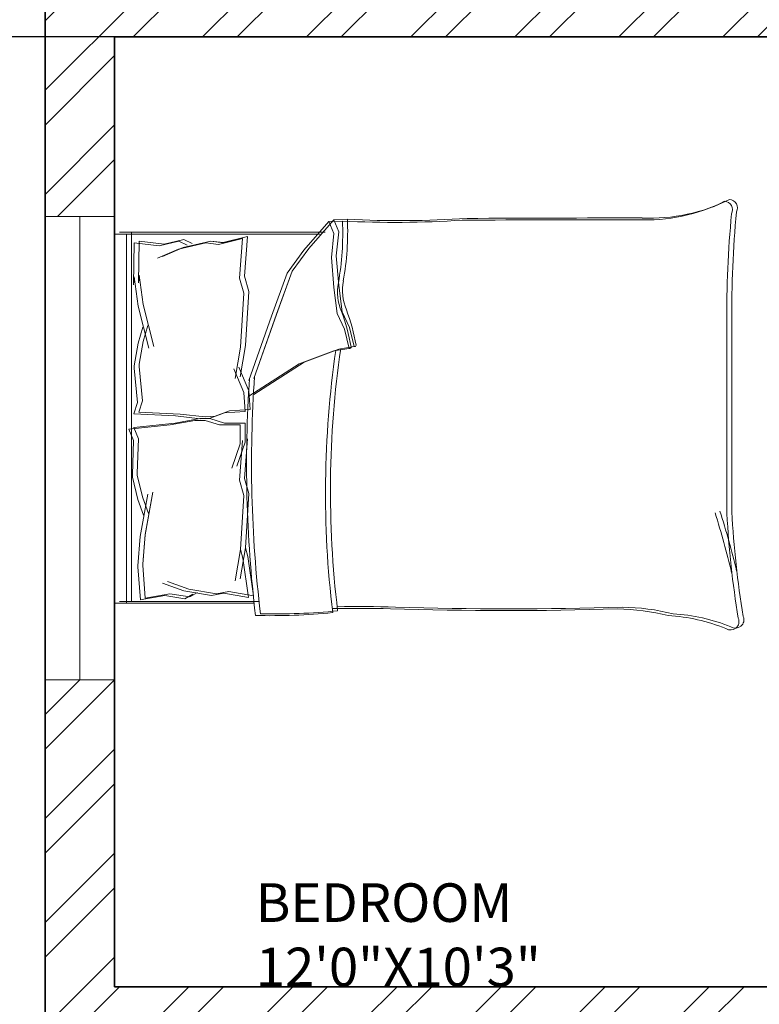
# Model space of a CAD drawing. Units: inches. Extents: x 2120 to 4013, y 1390 to 3019.
# Tile 5 of 59: x 2259 to 2355, y 1740 to 1868. Entities that reach past the tile are written whole.
import ezdxf

# ---------------------------------------------------------------- set-up
doc = ezdxf.new("R2010")
doc.units = ezdxf.units.IN
for name, color, linetype, lineweight in [('A-ANNO-DIMS', 2, 'Continuous', 18), ('A-AREA-IDEN', 7, 'Continuous', 18), ('A-FURN', 8, 'Continuous', 13), ('A-GLAZ', 4, 'Continuous', 18), ('A-WALL', 7, 'Continuous', 35), ('A-WALL-PATT', 252, 'Continuous', 13)]:
    doc.layers.add(name, color=color, linetype=linetype, lineweight=lineweight)
doc.styles.get("Standard").update_dxf_attribs({"font": 'arial.ttf'})
doc.dimstyles.get("Standard").update_dxf_attribs({"dimtxt": 0.18, "dimasz": 0.18, "dimexe": 0.18, "dimexo": 0.0625, "dimgap": 0.09, "dimtad": 0, "dimtih": 1, "dimtoh": 1, "dimdec": 4, "dimzin": 0, "dimdsep": 46, "dimtxsty": 'Standard', "dimcen": 0.09, "dimadec": 0, "dimazin": 0, "dimtfac": 1, "dimtdec": 4, "dimtofl": 0, "dimtmove": 0, "dimatfit": 3, "dimfxl": 1, "dimtolj": 1, "dimtzin": 0, "dimarcsym": 0})

# ---------------------------------------------------------------- blocks, each defined once
blk = doc.blocks.new('BED-DOUBLE-PLAN')
for p, q in [((3.48, 63.34), (3.48, 81.45)), ((3.48, 81.45), (51.27, 81.45)), ((3.7, 62.7), (3.7, 80.81)), ((51.27, 81.45), (51.27, 54.84)), ((51.5, 80.81), (51.5, 54.2)), ((3.48, 79.91), (51.27, 79.91)), ((3.7, 79.27), (51.5, 79.27)), ((16.88, 78.42), (19.77, 79.14)), ((19.77, 79.14), (20.09, 79.14)), ((20.09, 79.14), (24.54, 79)), ((24.54, 79), (25.98, 79.58)), ((25.98, 79.58), (26.56, 74.23)), ((3.9, 78.11), (8.18, 78.44)), ((3.9, 78.13), (4.47, 74.95)), ((4.13, 77.47), (8.41, 77.8)), ((8.18, 78.44), (8.29, 78.42)), ((8.29, 78.42), (12.11, 78.13)), ((8.41, 77.8), (8.51, 77.78)), ((8.51, 77.78), (12.34, 77.49)), ((12.11, 78.13), (17.6, 77.12)), ((14.86, 77.7), (16.88, 78.42)), ((15.08, 77.06), (17.11, 77.78)), ((17.11, 77.78), (20, 78.5)), ((20, 78.5), (20.32, 78.5)), ((20.32, 78.5), (24.77, 78.36)), ((24.77, 78.36), (26.21, 78.94)), ((26.21, 78.94), (26.79, 73.59)), ((27.98, 78.95), (27.73, 73.58)), ((28.21, 78.32), (27.96, 72.94)), ((29.46, 78.47), (27.98, 78.95)), ((29.69, 77.83), (28.21, 78.32)), ((33.89, 78.89), (29.46, 78.47)), ((34.11, 78.25), (29.69, 77.83)), ((34.21, 78.91), (33.89, 78.89)), ((34.43, 78.27), (34.11, 78.25)), ((37.14, 78.37), (34.21, 78.91)), ((37.37, 77.73), (34.43, 78.27)), ((41.92, 78.38), (36.5, 77.02)), ((39.2, 77.77), (37.14, 78.37)), ((45.71, 78.9), (41.92, 78.38)), ((45.94, 78.26), (42.14, 77.74)), ((50.11, 78.89), (44.71, 78.99)), ((44.71, 78.99), (45.71, 78.9)), ((50.34, 78.25), (44.94, 78.35)), ((44.94, 78.35), (45.94, 78.26)), ((50.11, 78.89), (49.73, 75.68)), ((50.34, 78.25), (49.96, 75.04)), ((4.12, 77.49), (4.7, 74.31)), ((12.34, 77.49), (17.83, 76.48)), ((42.14, 77.74), (36.72, 76.38)), ((39.43, 77.13), (37.37, 77.73)), ((5.05, 72.49), (6.06, 75.24)), ((49.31, 73.19), (48.13, 75.87)), ((49.54, 72.55), (48.36, 75.23)), ((49.73, 75.68), (50.33, 73.11)), ((4.47, 74.95), (4.04, 72.35)), ((4.7, 74.31), (4.27, 71.71)), ((5.28, 71.85), (6.29, 74.6)), ((26.56, 74.23), (27.14, 71.05)), ((49.96, 75.04), (50.56, 72.47)), ((26.79, 73.59), (27.37, 70.41)), ((27.73, 73.58), (27.36, 70.37)), ((27.96, 72.94), (27.58, 69.73)), ((50.11, 69.62), (49.31, 73.19)), ((50.33, 73.11), (49.82, 72.06)), ((4.04, 72.35), (4.62, 71.33)), ((4.27, 71.71), (4.85, 70.7)), ((4.47, 68.88), (5.05, 72.49)), ((4.7, 68.24), (5.28, 71.85)), ((50.34, 68.98), (49.54, 72.55)), ((50.56, 72.47), (50.04, 71.42)), ((27.14, 71.05), (27.14, 69.74)), ((27.36, 70.37), (27.44, 69.07)), ((27.37, 70.41), (27.37, 69.1)), ((4.76, 67.29), (4.47, 68.88)), ((27.14, 69.74), (26.56, 67.86)), ((27.37, 69.1), (26.79, 67.23)), ((27.44, 69.07), (28.13, 67.23)), ((27.58, 69.73), (27.67, 68.43)), ((49.92, 68.01), (50.11, 69.62)), ((50.15, 67.37), (50.34, 68.98)), ((4.99, 66.65), (4.7, 68.24)), ((26.56, 67.86), (26.56, 65.18)), ((27.67, 68.43), (28.36, 66.59)), ((50.7, 64.87), (49.92, 68.01)), ((4.19, 64.11), (4.76, 67.29)), ((4.41, 63.47), (4.99, 66.65)), ((26.79, 67.23), (26.79, 64.54)), ((28.13, 67.23), (28.3, 64.55)), ((28.36, 66.59), (28.53, 63.91)), ((50.93, 64.23), (50.15, 67.37)), ((6.38, 65.82), (10.42, 65.15)), ((6.61, 65.18), (10.64, 64.51)), ((10.42, 65.15), (9.28, 64.83)), ((10.42, 65.15), (17.43, 64.72)), ((17.43, 64.72), (19.39, 65.28)), ((19.39, 65.28), (24.52, 64.87)), ((24.1, 65.18), (20.96, 66.27)), ((24.33, 64.54), (21.19, 65.63)), ((26.56, 65.18), (24.1, 65.18)), ((30.75, 64.71), (33.82, 65.99)), ((30.98, 64.07), (34.05, 65.35)), ((32.57, 65.82), (36.6, 65.15)), ((32.79, 65.18), (36.83, 64.51)), ((36.6, 65.15), (43.61, 64.72)), ((43.61, 64.72), (45.57, 65.28)), ((45.57, 65.28), (50.7, 64.87)), ((9.28, 64.83), (4.19, 64.11)), ((9.51, 64.19), (4.41, 63.47)), ((10.64, 64.51), (9.51, 64.19)), ((10.64, 64.51), (17.65, 64.08)), ((17.65, 64.08), (19.61, 64.64)), ((19.61, 64.64), (24.75, 64.23)), ((26.79, 64.54), (24.33, 64.54)), ((28.3, 64.55), (30.75, 64.71)), ((28.53, 63.91), (30.98, 64.07)), ((30.26, 64.06), (34.45, 57.57)), ((40.65, 61.13), (32.31, 64.06)), ((36.83, 64.51), (43.84, 64.08)), ((43.84, 64.08), (45.8, 64.64)), ((45.8, 64.64), (50.93, 64.23)), ((30.49, 63.42), (34.68, 56.93)), ((40.87, 60.49), (32.54, 63.42)), ((46.22, 59.12), (40.65, 61.13)), ((46.45, 58.48), (40.87, 60.49)), ((49.16, 56.95), (46.22, 59.12)), ((34.45, 57.57), (36.15, 53.08)), ((49.39, 56.31), (46.45, 58.48)), ((34.68, 56.93), (36.38, 52.44)), ((52.87, 53.7), (49.16, 56.95)), ((53.1, 53.06), (49.39, 56.31)), ((51.33, 53.08), (52.87, 53.7)), ((52.95, 51.96), (52.87, 53.7, 3.87)), ((36.15, 53.08), (36.46, 51.07)), ((36.38, 52.44), (36.69, 50.43)), ((38.94, 51.69), (40.96, 52.62)), ((40.96, 52.62), (44.36, 53.08)), ((41.18, 51.98), (44.59, 52.44)), ((44.36, 53.08), (48.23, 53.39)), ((44.59, 52.44), (48.46, 52.75)), ((48.23, 53.39), (51.33, 53.08)), ((48.46, 52.75), (51.56, 52.44)), ((51.56, 52.44), (53.1, 53.06)), ((53.18, 51.32), (53.1, 53.06, 3.87)), ((36.46, 51.07), (38.94, 51.69)), ((36.69, 50.43), (39.17, 51.05)), ((39.17, 51.05), (41.18, 51.98)), ((15.06, 2.2), (39.68, 2.2)), ((15.29, 1.56), (39.91, 1.56))]:
    blk.add_line(p, q)
for centre, radius, start, end in [((21.36, -100.61), 164.97, 86.0865, 96.7821), ((85.16, 61.35), 83.31, 178.7218, 185.604), ((85.39, 60.71), 83.31, 178.7218, 185.604), ((21.59, -101.25), 164.97, 86.0865, 96.7821), ((17.76, -74.87), 129.02, 81.7845, 96.9006), ((17.99, -75.51), 129.02, 81.7845, 96.9006), ((-167.31, 50.27), 170.11, 358.4762, 1.0082), ((-167.08, 49.63), 170.11, 358.4762, 1.0082), ((43.74, 46.38), 6.22, 78.6608, 113.7384), ((51.33, 88.1), 36.18, 259.8763, 272.5657), ((36.64, 51.01), 0.185, 160.2464, 271.1377), ((31.16, 79.96), 29.65, 280.6617, 289.8806), ((31.38, 79.32), 29.65, 280.6617, 289.8806), ((43.97, 45.74), 6.22, 78.6608, 113.7384), ((51.56, 87.46), 36.18, 259.8763, 272.5657), ((182.27, 45.13), 129.5, 176.9791, 183.8365), ((182.5, 44.49), 129.5, 176.9791, 183.8365), ((36.87, 50.37), 0.185, 160.2464, 271.1377), ((484.82, 30.83), 482.31, 178.2277, 181.7185), ((485.05, 30.19), 482.31, 178.2277, 181.7185), ((-4508.74, 13.62), 4561.86, 0.00217, 0.28689), ((-4508.51, 12.99), 4561.86, 0.00217, 0.28689), ((-26.9, 16.93), 29.63, 346.0648, 358.9113), ((-26.67, 16.29), 29.63, 346.0648, 358.9113), ((76.16, 12.78), 23.07, 177.4714, 206.4681), ((76.39, 12.14), 23.07, 177.4714, 206.4681), ((-21.66, 11.17), 23.56, 337.9751, 356.652), ((-21.43, 10.53), 23.56, 337.9751, 356.652), ((-17.22, 105.16), 106.46, 283.3832, 287.7053), ((-16.99, 104.52), 106.46, 283.3832, 287.7053), ((1.09, 1.73), 1.09, 146.1736, 293.4781), ((1.32, 1.09), 1.09, 146.1736, 293.4781), ((21.43, -119.39), 121.76, 92.9958, 99.4091), ((21.66, -120.03), 121.76, 92.9958, 99.4091), ((41.15, -130.83), 133.04, 84.4998, 90.6351), ((41.38, -131.47), 133.04, 84.4998, 90.6351), ((54.41, 2.58), 1.1, 242.6588, 356.02), ((54.64, 1.94), 1.1, 242.6588, 356.02)]:
    blk.add_arc(centre, radius, start, end)
blk = doc.blocks.new('WIN-PLAN-60IN-02')
for p, q in [((0, 0), (0, 9)), ((0, 9), (0, 4.5)), ((60, 4.5), (60, 9)), ((60, 9), (60, 0)), ((0, 4.5), (60, 4.5))]:
    blk.add_line(p, q)
blk = doc.blocks.new('*D213')
at = {"layer": 'A-ANNO-DIMS', "color": 0, "lineweight": -2, "transparency": 16777216}
for p, q in [((2271.67, 1865.53), (2217.55, 1865.53)), ((2217.73, 1865.35), (2217.73, 1723.71)), ((2217.73, 1581.71), (2217.73, 1723.35)), ((2262.67, 1581.53), (2217.55, 1581.53))]:
    blk.add_line(p, q, dxfattribs=at)
at = {"layer": 'A-ANNO-DIMS', "color": 0, "transparency": 16777216}
for points in [[(2217.7, 1865.35), (2217.76, 1865.35), (2217.73, 1865.53)], [(2217.7, 1581.71), (2217.76, 1581.71), (2217.73, 1581.53)]]:
    blk.add_solid(points, dxfattribs=at)
at = {"layer": 'Defpoints', "color": 0, "transparency": 16777216}
for p in [(2217.73, 1865.53), (2271.73, 1865.53), (2262.73, 1581.53)]:
    blk.add_point(p, dxfattribs=at)
at = {"layer": 'A-ANNO-DIMS', "color": 0, "transparency": 16777216, "insert": (2217.73, 1723.53), "char_height": 0.18, "attachment_point": 5}
blk.add_mtext('\\A1;284', dxfattribs=at)
blk = doc.blocks.new('*D214')
at = {"layer": 'A-ANNO-DIMS', "color": 0, "lineweight": -2, "transparency": 16777216}
for p, q in [((2271.67, 2075.03), (2217.55, 2075.03)), ((2217.73, 2074.85), (2217.73, 1970.46)), ((2217.73, 1865.71), (2217.73, 1970.1)), ((2271.67, 1865.53), (2217.55, 1865.53))]:
    blk.add_line(p, q, dxfattribs=at)
at = {"layer": 'A-ANNO-DIMS', "color": 0, "transparency": 16777216}
for points in [[(2217.7, 2074.85), (2217.76, 2074.85), (2217.73, 2075.03)], [(2217.7, 1865.71), (2217.76, 1865.71), (2217.73, 1865.53)]]:
    blk.add_solid(points, dxfattribs=at)
at = {"layer": 'Defpoints', "color": 0, "transparency": 16777216}
for p in [(2217.73, 2075.03), (2271.73, 2075.03), (2271.73, 1865.53)]:
    blk.add_point(p, dxfattribs=at)
at = {"layer": 'A-ANNO-DIMS', "color": 0, "transparency": 16777216, "insert": (2217.73, 1970.28), "char_height": 0.18, "attachment_point": 5}
blk.add_mtext('\\A1;209.5', dxfattribs=at)

msp = doc.modelspace()

# ---------------------------------------------------------------- hatches: boundary and pattern name
at = {"layer": 'A-WALL-PATT'}
h = msp.add_hatch(dxfattribs=at)
h.set_pattern_fill('ANSI32', color=256)
h.paths.add_polyline_path([(2271.7331, 2343.531), (2283.3788, 2343.531), (2283.3788, 2348.031), (2283.3788, 2352.5306), (2262.7331, 2352.5306), (2262.7331, 2182.638), (2267.2331, 2182.638), (2271.7331, 2182.638), (2271.7331, 2219.031), (2391.7331, 2219.031), (2391.7331, 2214.189), (2393.9831, 2214.189), (2396.2331, 2214.189), (2396.2331, 2219.031), (2420.2331, 2219.031), (2420.2331, 2225.7535), (2417.2197, 2225.7535), (2415.7331, 2225.7535), (2415.7331, 2223.5306), (2271.7331, 2223.5306)])
h.paths.add_polyline_path([(2380.0942, 2352.5306), (2343.3788, 2352.5306), (2343.3788, 2343.531), (2363.2331, 2343.531), (2363.2331, 2288.8489), (2365.4831, 2288.8489), (2367.7331, 2288.8489), (2367.7331, 2343.531), (2380.0942, 2343.531)], flags=17)
h.paths.add_polyline_path([(2432.4339, 2352.5306), (2404.0943, 2352.5306), (2404.0943, 2343.531), (2415.7331, 2343.531), (2415.7331, 2264.0306), (2367.7331, 2264.0306), (2367.7331, 2266.4872), (2363.2331, 2266.4872), (2363.2331, 2259.531), (2367.7331, 2259.531), (2415.7331, 2259.531), (2415.7331, 2255.0658), (2420.2331, 2255.0658), (2420.2331, 2259.531), (2424.5717, 2259.531), (2424.5717, 2261.781), (2424.5717, 2264.0306), (2420.2331, 2264.0306), (2420.2331, 2343.531), (2432.4339, 2343.531)])
h.paths.add_polyline_path([(2508.9115, 2352.5306), (2456.4339, 2352.5306), (2456.4339, 2343.531), (2468.2331, 2343.531), (2468.2331, 2264.0306), (2448.0487, 2264.0306), (2448.0487, 2259.531), (2468.2331, 2259.531), (2468.2331, 2255.5496), (2472.7331, 2255.5496), (2472.7331, 2343.531), (2508.9115, 2343.531)])
h.paths.add_polyline_path([(2637.7331, 2352.5306), (2544.9116, 2352.5306), (2544.9116, 2343.531), (2589.7331, 2343.531), (2633.2331, 2343.531), (2637.7331, 2343.531)])
h.paths.add_polyline_path([(2594.2331, 2343.5306), (2589.7331, 2343.5306), (2589.7331, 2259.5306), (2589.7331, 2252.4915), (2591.9831, 2252.4915), (2594.2331, 2252.4915)])
h.paths.add_polyline_path([(2637.7331, 2223.5306), (2594.2331, 2223.5306), (2594.2331, 2230.1988), (2591.9831, 2230.1988), (2589.7331, 2230.1988), (2589.7331, 2223.5306), (2472.7331, 2223.5306), (2468.2331, 2223.5306), (2468.2331, 2219.031), (2628.7331, 2219.031), (2628.7331, 2138.031), (2637.7331, 2138.031)])
h.paths.add_polyline_path([(3822.6535, 2458.4402), (3874.9468, 2458.4402), (3874.9468, 2476.9866), (3822.6535, 2476.9866)], flags=9)
h.paths.add_polyline_path([(3834.6921, 2781.8174), (3935.9206, 2781.8174), (3935.9206, 2800.3638), (3834.6921, 2800.3638)], flags=9)
h.paths.add_polyline_path([(3832.2843, 2837.9683), (3884.5776, 2837.9683), (3884.5776, 2856.5146), (3832.2843, 2856.5146)], flags=9)
h.paths.add_polyline_path([(3830.9388, 2861.4782), (3956.8958, 2861.4782), (3956.8958, 2880.0245), (3830.9388, 2880.0245)], flags=9)
h.paths.add_polyline_path([(3870.6966, 2352.5752), (3887.9272, 2352.5752), (3887.9272, 2377.3037), (3870.6966, 2377.3037)], flags=9)
h.paths.add_polyline_path([(3289.2701, 2413.161), (3435.2223, 2413.161), (3435.2223, 2450.2538), (3289.2701, 2450.2538)], flags=9)
h.paths.add_polyline_path([(2487.6944, 2414.3601), (2637.8335, 2414.3601), (2637.8335, 2451.4528), (2487.6944, 2451.4528)], flags=9)
h.paths.add_polyline_path([(2567.3724, 1457.9199), (2815.296, 1457.9199), (2815.296, 1495.0127), (2567.3724, 1495.0127)], flags=9)
h.paths.add_polyline_path([(2655.3825, 2093.2363), (2685.9555, 2093.2363), (2685.9555, 2111.8937), (2655.3825, 2111.8937)], flags=9)
h.paths.add_polyline_path([(2543.9218, 1550.6671), (2587.8406, 1550.6671), (2587.8406, 1569.3244), (2543.9218, 1569.3244)], flags=9)
h.paths.add_polyline_path([(2905.1384, 1543.8113), (2949.0572, 1543.8113), (2949.0572, 1562.4686), (2905.1384, 1562.4686)], flags=9)
h.paths.add_polyline_path([(2736.4118, 1702.4736), (2784.2153, 1702.4736), (2784.2153, 1721.1309), (2736.4118, 1721.1309)], flags=9)
h.paths.add_polyline_path([(2912.8666, 1710.4168), (2951.707, 1710.4168), (2951.707, 1729.0741), (2912.8666, 1729.0741)], flags=9)
h.paths.add_polyline_path([(2923.5785, 1763.5038), (2959.7279, 1763.5038), (2959.7279, 1782.1611), (2923.5785, 1782.1611)], flags=9)
h.paths.add_polyline_path([(2925.2114, 1809.6137), (2967.1861, 1809.6137), (2967.1861, 1828.271), (2925.2114, 1828.271)], flags=9)
h.paths.add_polyline_path([(2996.2711, 1878.9003), (2996.2711, 1913.109), (2977.6138, 1913.109), (2977.6138, 1878.9003)], flags=9)
h.paths.add_polyline_path([(2883.0859, 1895.7192), (2927.1855, 1895.7192), (2927.1855, 1914.3766), (2883.0859, 1914.3766)], flags=9)
h.paths.add_polyline_path([(2787.3924, 1810.8013), (2841.0213, 1810.8013), (2841.0213, 1829.4587), (2787.3924, 1829.4587)], flags=9)
h.paths.add_polyline_path([(2775.6399, 2101.7395), (2829.2689, 2101.7395), (2829.2689, 2120.3968), (2775.6399, 2120.3968)], flags=9)
h.paths.add_polyline_path([(2913.0263, 2075.817), (2951.8667, 2075.817), (2951.8667, 2094.4744), (2913.0263, 2094.4744)], flags=9)
h.paths.add_polyline_path([(2929.966, 2133.3669), (2966.1154, 2133.3669), (2966.1154, 2152.0243), (2929.966, 2152.0243)], flags=9)
h.paths.add_polyline_path([(2932.7502, 2182.6088), (2968.8996, 2182.6088), (2968.8996, 2201.2662), (2932.7502, 2201.2662)], flags=9)
h.paths.add_polyline_path([(2996.0681, 2266.3173), (2996.0681, 2300.5261), (2977.4108, 2300.5261), (2977.4108, 2266.3173)], flags=9)
h.paths.add_polyline_path([(2885.1039, 2279.2186), (2929.2035, 2279.2186), (2929.2035, 2297.8759), (2885.1039, 2297.8759)], flags=9)
h.paths.add_polyline_path([(2735.7042, 2218.3197), (2783.5078, 2218.3197), (2783.5078, 2236.9771), (2735.7042, 2236.9771)], flags=9)
h.paths.add_polyline_path([(2635.6049, 2044.0085), (2648.9678, 2044.0085), (2648.9678, 2054.312), (2635.6049, 2054.312)], flags=9)
h.paths.add_polyline_path([(2714.0148, 1923.0473), (2727.3777, 1923.0473), (2727.3777, 1933.3508), (2714.0148, 1933.3508)], flags=9)
h.paths.add_polyline_path([(2709.0345, 1988.1628), (2722.3974, 1988.1628), (2722.3974, 1998.4663), (2709.0345, 1998.4663)], flags=9)
h.paths.add_polyline_path([(2592.8935, 1962.1763), (2606.2564, 1962.1763), (2606.2564, 1972.4799), (2592.8935, 1972.4799)], flags=9)
h.paths.add_polyline_path([(2618.3996, 1985.9724), (2644.1942, 1985.9724), (2644.1942, 1996.2759), (2618.3996, 1996.2759)], flags=9)
h.paths.add_polyline_path([(2601.279, 1920.5869), (2614.6419, 1920.5869), (2614.6419, 1930.8904), (2601.279, 1930.8904)], flags=9)
h.paths.add_polyline_path([(2692.3278, 1932.7645), (2704.5311, 1932.7645), (2704.5311, 1943.0681), (2692.3278, 1943.0681)], flags=9)
h.paths.add_polyline_path([(2311.122, 1672.7318), (2355.0408, 1672.7318), (2355.0408, 1691.3892), (2311.122, 1691.3892)], flags=9)
h.paths.add_polyline_path([(2456.2551, 1632.3198), (2492.4796, 1632.3198), (2492.4796, 1650.9772), (2456.2551, 1650.9772)], flags=9)
h.paths.add_polyline_path([(2401.0766, 1631.4793), (2437.301, 1631.4793), (2437.301, 1650.1367), (2401.0766, 1650.1367)], flags=9)
h.paths.add_polyline_path([(2546.7054, 1700.9235), (2594.509, 1700.9235), (2594.509, 1719.5809), (2546.7054, 1719.5809)], flags=9)
h.paths.add_polyline_path([(2445.4866, 1766.9937), (2497.5261, 1766.9937), (2497.5261, 1785.651), (2445.4866, 1785.651)], flags=9)
h.paths.add_polyline_path([(2287.9992, 1739.7675), (2326.8396, 1739.7675), (2326.8396, 1758.4248), (2287.9992, 1758.4248)], flags=9)
h.paths.add_polyline_path([(2458.5279, 1924.7607), (2510.5675, 1924.7607), (2510.5675, 1943.4181), (2458.5279, 1943.4181)], flags=9)
h.paths.add_polyline_path([(2309.2811, 1902.7642), (2345.4305, 1902.7642), (2345.4305, 1921.4215), (2309.2811, 1921.4215)], flags=9)
h.paths.add_polyline_path([(2490.7554, 2018.9392), (2530.7896, 2018.9392), (2530.7896, 2037.5965), (2490.7554, 2037.5965)], flags=9)
h.paths.add_polyline_path([(2402.143, 2024.7393), (2438.5414, 2024.7393), (2438.5414, 2043.3966), (2402.143, 2043.3966)], flags=9)
h.paths.add_polyline_path([(2287.856, 1931.7926), (2326.6964, 1931.7926), (2326.6964, 1950.4499), (2287.856, 1950.4499)], flags=9)
h.paths.add_polyline_path([(2281.7979, 2193.5771), (2320.6383, 2193.5771), (2320.6383, 2212.2344), (2281.7979, 2212.2344)], flags=25)
h.paths.add_polyline_path([(2484.0754, 2093.892), (2536.115, 2093.892), (2536.115, 2112.5494), (2484.0754, 2112.5494)], flags=9)
h.paths.add_polyline_path([(2624.7948, 2281.8639), (2624.7948, 2311.4137), (2606.1375, 2311.4137), (2606.1375, 2281.8639)], flags=9)
h.paths.add_polyline_path([(2507.5036, 2290.3639), (2541.934, 2290.3639), (2541.934, 2309.0212), (2507.5036, 2309.0212)], flags=9)
h.paths.add_polyline_path([(2423.1076, 2285.2202), (2459.332, 2285.2202), (2459.332, 2303.8776), (2423.1076, 2303.8776)], flags=9)
h.paths.add_polyline_path([(2374.5467, 2289.6272), (2410.7711, 2289.6272), (2410.7711, 2308.2846), (2374.5467, 2308.2846)], flags=25)
h.paths.add_polyline_path([(2277.4907, 2227.5651), (2316.3311, 2227.5651), (2316.3311, 2246.2224), (2277.4907, 2246.2224)], flags=25)
h.paths.add_polyline_path([(2655.3825, 2093.2367), (2685.9555, 2093.2367), (2685.9555, 2111.894), (2655.3825, 2111.894)], flags=9)
h.paths.add_polyline_path([(2543.9217, 1550.6674), (2587.8406, 1550.6674), (2587.8406, 1569.3247), (2543.9217, 1569.3247)], flags=9)
h.paths.add_polyline_path([(2905.1384, 1543.8116), (2949.0572, 1543.8116), (2949.0572, 1562.4689), (2905.1384, 1562.4689)], flags=9)
h.paths.add_polyline_path([(2736.4118, 1702.4739), (2784.2153, 1702.4739), (2784.2153, 1721.1312), (2736.4118, 1721.1312)], flags=9)
h.paths.add_polyline_path([(2912.8666, 1710.4171), (2951.707, 1710.4171), (2951.707, 1729.0744), (2912.8666, 1729.0744)], flags=9)
h.paths.add_polyline_path([(2923.5785, 1763.5041), (2959.7279, 1763.5041), (2959.7279, 1782.1614), (2923.5785, 1782.1614)], flags=9)
h.paths.add_polyline_path([(2925.2114, 1809.614), (2967.1861, 1809.614), (2967.1861, 1828.2713), (2925.2114, 1828.2713)], flags=9)
h.paths.add_polyline_path([(2996.2711, 1878.9006), (2996.2711, 1913.1094), (2977.6137, 1913.1094), (2977.6137, 1878.9006)], flags=9)
h.paths.add_polyline_path([(2883.0859, 1895.7195), (2927.1855, 1895.7195), (2927.1855, 1914.3769), (2883.0859, 1914.3769)], flags=9)
h.paths.add_polyline_path([(2787.3924, 1810.8016), (2841.0213, 1810.8016), (2841.0213, 1829.459), (2787.3924, 1829.459)], flags=9)
h.paths.add_polyline_path([(2775.6399, 2101.7398), (2829.2688, 2101.7398), (2829.2688, 2120.3971), (2775.6399, 2120.3971)], flags=9)
h.paths.add_polyline_path([(2913.0263, 2075.8173), (2951.8667, 2075.8173), (2951.8667, 2094.4747), (2913.0263, 2094.4747)], flags=9)
h.paths.add_polyline_path([(2929.966, 2133.3672), (2966.1154, 2133.3672), (2966.1154, 2152.0246), (2929.966, 2152.0246)], flags=9)
h.paths.add_polyline_path([(2932.7502, 2182.6091), (2968.8996, 2182.6091), (2968.8996, 2201.2665), (2932.7502, 2201.2665)], flags=9)
h.paths.add_polyline_path([(2996.0681, 2266.3176), (2996.0681, 2300.5264), (2977.4108, 2300.5264), (2977.4108, 2266.3176)], flags=9)
h.paths.add_polyline_path([(2885.1039, 2279.2189), (2929.2035, 2279.2189), (2929.2035, 2297.8762), (2885.1039, 2297.8762)], flags=9)
h.paths.add_polyline_path([(2735.7042, 2218.32), (2783.5078, 2218.32), (2783.5078, 2236.9774), (2735.7042, 2236.9774)], flags=9)
h.paths.add_polyline_path([(2635.6048, 2044.0088), (2648.9677, 2044.0088), (2648.9677, 2054.3123), (2635.6048, 2054.3123)], flags=9)
h.paths.add_polyline_path([(2714.0148, 1923.0476), (2727.3777, 1923.0476), (2727.3777, 1933.3511), (2714.0148, 1933.3511)], flags=9)
h.paths.add_polyline_path([(2709.0345, 1988.1631), (2722.3974, 1988.1631), (2722.3974, 1998.4666), (2709.0345, 1998.4666)], flags=9)
h.paths.add_polyline_path([(2592.8935, 1962.1766), (2606.2564, 1962.1766), (2606.2564, 1972.4802), (2592.8935, 1972.4802)], flags=9)
h.paths.add_polyline_path([(2618.3995, 1985.9727), (2644.1942, 1985.9727), (2644.1942, 1996.2762), (2618.3995, 1996.2762)], flags=9)
h.paths.add_polyline_path([(2601.279, 1920.5872), (2614.6419, 1920.5872), (2614.6419, 1930.8908), (2601.279, 1930.8908)], flags=9)
h.paths.add_polyline_path([(2692.3278, 1932.7648), (2704.5311, 1932.7648), (2704.5311, 1943.0684), (2692.3278, 1943.0684)], flags=9)
h.paths.add_polyline_path([(2311.122, 1672.7321), (2355.0408, 1672.7321), (2355.0408, 1691.3895), (2311.122, 1691.3895)], flags=9)
h.paths.add_polyline_path([(2456.2551, 1632.3201), (2492.4795, 1632.3201), (2492.4795, 1650.9775), (2456.2551, 1650.9775)], flags=9)
h.paths.add_polyline_path([(2401.0766, 1631.4796), (2437.301, 1631.4796), (2437.301, 1650.137), (2401.0766, 1650.137)], flags=9)
h.paths.add_polyline_path([(2546.7054, 1700.9238), (2594.509, 1700.9238), (2594.509, 1719.5812), (2546.7054, 1719.5812)], flags=9)
h.paths.add_polyline_path([(2445.4866, 1766.994), (2497.5261, 1766.994), (2497.5261, 1785.6513), (2445.4866, 1785.6513)], flags=9)
h.paths.add_polyline_path([(2287.9992, 1739.7678), (2326.8396, 1739.7678), (2326.8396, 1758.4251), (2287.9992, 1758.4251)], flags=9)
h.paths.add_polyline_path([(2458.5279, 1924.7611), (2510.5675, 1924.7611), (2510.5675, 1943.4184), (2458.5279, 1943.4184)], flags=9)
h.paths.add_polyline_path([(2309.2811, 1902.7645), (2345.4305, 1902.7645), (2345.4305, 1921.4218), (2309.2811, 1921.4218)], flags=9)
h.paths.add_polyline_path([(2490.7554, 2018.9395), (2530.7895, 2018.9395), (2530.7895, 2037.5968), (2490.7554, 2037.5968)], flags=9)
h.paths.add_polyline_path([(2402.143, 2024.7396), (2438.5413, 2024.7396), (2438.5413, 2043.3969), (2402.143, 2043.3969)], flags=9)
h.paths.add_polyline_path([(2287.856, 1931.7929), (2326.6964, 1931.7929), (2326.6964, 1950.4502), (2287.856, 1950.4502)], flags=9)
h.paths.add_polyline_path([(2281.7979, 2193.5774), (2320.6383, 2193.5774), (2320.6383, 2212.2347), (2281.7979, 2212.2347)], flags=25)
h.paths.add_polyline_path([(2484.0754, 2093.8924), (2536.115, 2093.8924), (2536.115, 2112.5497), (2484.0754, 2112.5497)], flags=9)
h.paths.add_polyline_path([(2624.7948, 2281.8642), (2624.7948, 2311.414), (2606.1374, 2311.414), (2606.1374, 2281.8642)], flags=9)
h.paths.add_polyline_path([(2507.5035, 2290.3642), (2541.934, 2290.3642), (2541.934, 2309.0215), (2507.5035, 2309.0215)], flags=9)
h.paths.add_polyline_path([(2423.1075, 2285.2205), (2459.332, 2285.2205), (2459.332, 2303.8779), (2423.1075, 2303.8779)], flags=9)
h.paths.add_polyline_path([(2374.5467, 2289.6275), (2410.7711, 2289.6275), (2410.7711, 2308.2849), (2374.5467, 2308.2849)], flags=25)
h.paths.add_polyline_path([(2277.4907, 2227.5654), (2316.3311, 2227.5654), (2316.3311, 2246.2227), (2277.4907, 2246.2227)], flags=25)
h = msp.add_hatch(dxfattribs=at)
h.set_pattern_fill('ANSI32', color=256)
h.paths.add_polyline_path([(2271.7331, 1980.389), (2262.7331, 1980.389), (2262.7331, 1912.8434), (2267.2331, 1912.8434), (2271.7331, 1912.8434), (2271.7331, 1922.531), (2351.2331, 1922.531), (2351.2331, 1901.4728), (2355.7331, 1901.4728), (2355.7331, 1922.531), (2357.9815, 1922.531), (2357.9815, 1926.5306), (2271.7331, 1926.5306)])
h.paths.add_polyline_path([(2589.2331, 1949.1622), (2584.7331, 1949.1622), (2580.2331, 1949.1622), (2580.2331, 1874.5306), (2355.7331, 1874.5306), (2355.7331, 1880.1922), (2351.2331, 1880.1922), (2351.2331, 1874.5306), (2271.7331, 1874.5306), (2271.7331, 1888.8431), (2262.7331, 1888.8431), (2262.7331, 1842.2909), (2267.2331, 1842.2909), (2271.7331, 1842.2909), (2271.7331, 1865.531), (2415.7331, 1865.531), (2415.7331, 1779.7286), (2420.2331, 1779.7286), (2420.2331, 1865.531), (2589.2331, 1865.531)])
h.paths.add_polyline_path([(2271.7331, 1782.2906), (2262.7331, 1782.2906), (2262.7331, 1711.4639), (2267.2331, 1711.4639), (2271.7331, 1711.4639), (2271.7331, 1738.031), (2420.2331, 1738.031), (2420.2331, 1742.531), (2420.2331, 1747.3376), (2417.9831, 1747.3376), (2415.7331, 1747.3376), (2415.7331, 1742.5306), (2271.7331, 1742.5306)])
h.paths.add_polyline_path([(2271.7331, 1627.031), (2362.3957, 1627.031), (2362.3957, 1629.281), (2362.3957, 1631.5306), (2271.7331, 1631.5306), (2271.7331, 1675.4636), (2262.7331, 1675.4636), (2262.7331, 1581.531), (2405.3032, 1581.531), (2405.3032, 1586.031), (2405.3032, 1590.5306), (2396.2331, 1590.5306), (2396.2331, 1691.4513), (2418.7206, 1691.4513), (2418.7206, 1695.951), (2396.2331, 1695.951), (2391.7331, 1695.951), (2391.7331, 1631.5306), (2386.7425, 1631.5306), (2386.7425, 1629.2806), (2386.7425, 1627.031), (2391.7331, 1627.031), (2391.7331, 1586.1709), (2271.7331, 1586.1709)])
h.paths.add_polyline_path([(2459.6703, 1590.5306), (2429.3032, 1590.5306), (2429.3032, 1581.531), (2459.6703, 1581.531), (2459.6703, 1586.031)])
h.paths.add_polyline_path([(2501.2331, 1590.531), (2501.2331, 1665.0195), (2498.9831, 1665.0195), (2496.7331, 1665.0195), (2496.7331, 1590.5306), (2483.8201, 1590.5306), (2483.8201, 1590.1579), (2483.6704, 1590.1579), (2483.6704, 1581.531), (2505.0196, 1581.531), (2505.0196, 1583.781), (2505.0196, 1586.0306), (2501.2331, 1586.0306)])
h.paths.add_polyline_path([(2544.1361, 1583.781), (2544.1361, 1586.0306), (2527.1368, 1586.0306), (2527.1368, 1583.7806), (2527.1368, 1581.531), (2544.1361, 1581.531)])
h.paths.add_polyline_path([(3822.6535, 2458.4402), (3874.9468, 2458.4402), (3874.9468, 2476.9866), (3822.6535, 2476.9866)], flags=9)
h.paths.add_polyline_path([(3834.6921, 2781.8174), (3935.9206, 2781.8174), (3935.9206, 2800.3638), (3834.6921, 2800.3638)], flags=9)
h.paths.add_polyline_path([(3832.2843, 2837.9683), (3884.5776, 2837.9683), (3884.5776, 2856.5146), (3832.2843, 2856.5146)], flags=9)
h.paths.add_polyline_path([(3830.9388, 2861.4782), (3956.8958, 2861.4782), (3956.8958, 2880.0245), (3830.9388, 2880.0245)], flags=9)
h.paths.add_polyline_path([(3870.6966, 2352.5752), (3887.9272, 2352.5752), (3887.9272, 2377.3037), (3870.6966, 2377.3037)], flags=9)
h.paths.add_polyline_path([(3289.2701, 2413.161), (3435.2223, 2413.161), (3435.2223, 2450.2538), (3289.2701, 2450.2538)], flags=9)
h.paths.add_polyline_path([(2487.6944, 2414.3601), (2637.8335, 2414.3601), (2637.8335, 2451.4528), (2487.6944, 2451.4528)], flags=9)
h.paths.add_polyline_path([(2567.3724, 1457.9199), (2815.296, 1457.9199), (2815.296, 1495.0127), (2567.3724, 1495.0127)], flags=9)
h.paths.add_polyline_path([(2655.3825, 2093.2363), (2685.9555, 2093.2363), (2685.9555, 2111.8937), (2655.3825, 2111.8937)], flags=9)
h.paths.add_polyline_path([(2543.9218, 1550.6671), (2587.8406, 1550.6671), (2587.8406, 1569.3244), (2543.9218, 1569.3244)], flags=9)
h.paths.add_polyline_path([(2905.1384, 1543.8113), (2949.0572, 1543.8113), (2949.0572, 1562.4686), (2905.1384, 1562.4686)], flags=9)
h.paths.add_polyline_path([(2736.4118, 1702.4736), (2784.2153, 1702.4736), (2784.2153, 1721.1309), (2736.4118, 1721.1309)], flags=9)
h.paths.add_polyline_path([(2912.8666, 1710.4168), (2951.707, 1710.4168), (2951.707, 1729.0741), (2912.8666, 1729.0741)], flags=9)
h.paths.add_polyline_path([(2923.5785, 1763.5038), (2959.7279, 1763.5038), (2959.7279, 1782.1611), (2923.5785, 1782.1611)], flags=9)
h.paths.add_polyline_path([(2925.2114, 1809.6137), (2967.1861, 1809.6137), (2967.1861, 1828.271), (2925.2114, 1828.271)], flags=9)
h.paths.add_polyline_path([(2996.2711, 1878.9003), (2996.2711, 1913.109), (2977.6138, 1913.109), (2977.6138, 1878.9003)], flags=9)
h.paths.add_polyline_path([(2883.0859, 1895.7192), (2927.1855, 1895.7192), (2927.1855, 1914.3766), (2883.0859, 1914.3766)], flags=9)
h.paths.add_polyline_path([(2787.3924, 1810.8013), (2841.0213, 1810.8013), (2841.0213, 1829.4587), (2787.3924, 1829.4587)], flags=9)
h.paths.add_polyline_path([(2775.6399, 2101.7395), (2829.2689, 2101.7395), (2829.2689, 2120.3968), (2775.6399, 2120.3968)], flags=9)
h.paths.add_polyline_path([(2913.0263, 2075.817), (2951.8667, 2075.817), (2951.8667, 2094.4744), (2913.0263, 2094.4744)], flags=9)
h.paths.add_polyline_path([(2929.966, 2133.3669), (2966.1154, 2133.3669), (2966.1154, 2152.0243), (2929.966, 2152.0243)], flags=9)
h.paths.add_polyline_path([(2932.7502, 2182.6088), (2968.8996, 2182.6088), (2968.8996, 2201.2662), (2932.7502, 2201.2662)], flags=9)
h.paths.add_polyline_path([(2996.0681, 2266.3173), (2996.0681, 2300.5261), (2977.4108, 2300.5261), (2977.4108, 2266.3173)], flags=9)
h.paths.add_polyline_path([(2885.1039, 2279.2186), (2929.2035, 2279.2186), (2929.2035, 2297.8759), (2885.1039, 2297.8759)], flags=9)
h.paths.add_polyline_path([(2735.7042, 2218.3197), (2783.5078, 2218.3197), (2783.5078, 2236.9771), (2735.7042, 2236.9771)], flags=9)
h.paths.add_polyline_path([(2635.6049, 2044.0085), (2648.9678, 2044.0085), (2648.9678, 2054.312), (2635.6049, 2054.312)], flags=9)
h.paths.add_polyline_path([(2714.0148, 1923.0473), (2727.3777, 1923.0473), (2727.3777, 1933.3508), (2714.0148, 1933.3508)], flags=9)
h.paths.add_polyline_path([(2709.0345, 1988.1628), (2722.3974, 1988.1628), (2722.3974, 1998.4663), (2709.0345, 1998.4663)], flags=9)
h.paths.add_polyline_path([(2592.8935, 1962.1763), (2606.2564, 1962.1763), (2606.2564, 1972.4799), (2592.8935, 1972.4799)], flags=9)
h.paths.add_polyline_path([(2618.3996, 1985.9724), (2644.1942, 1985.9724), (2644.1942, 1996.2759), (2618.3996, 1996.2759)], flags=9)
h.paths.add_polyline_path([(2601.279, 1920.5869), (2614.6419, 1920.5869), (2614.6419, 1930.8904), (2601.279, 1930.8904)], flags=9)
h.paths.add_polyline_path([(2692.3278, 1932.7645), (2704.5311, 1932.7645), (2704.5311, 1943.0681), (2692.3278, 1943.0681)], flags=9)
h.paths.add_polyline_path([(2311.122, 1672.7318), (2355.0408, 1672.7318), (2355.0408, 1691.3892), (2311.122, 1691.3892)], flags=25)
h.paths.add_polyline_path([(2456.2551, 1632.3198), (2492.4796, 1632.3198), (2492.4796, 1650.9772), (2456.2551, 1650.9772)], flags=9)
h.paths.add_polyline_path([(2401.0766, 1631.4793), (2437.301, 1631.4793), (2437.301, 1650.1367), (2401.0766, 1650.1367)], flags=9)
h.paths.add_polyline_path([(2546.7054, 1700.9235), (2594.509, 1700.9235), (2594.509, 1719.5809), (2546.7054, 1719.5809)], flags=9)
h.paths.add_polyline_path([(2445.4866, 1766.9937), (2497.5261, 1766.9937), (2497.5261, 1785.651), (2445.4866, 1785.651)], flags=9)
h.paths.add_polyline_path([(2287.9992, 1739.7675), (2326.8396, 1739.7675), (2326.8396, 1758.4248), (2287.9992, 1758.4248)], flags=24)
h.paths.add_polyline_path([(2458.5279, 1924.7607), (2510.5675, 1924.7607), (2510.5675, 1943.4181), (2458.5279, 1943.4181)], flags=25)
h.paths.add_polyline_path([(2309.2811, 1902.7642), (2345.4305, 1902.7642), (2345.4305, 1921.4215), (2309.2811, 1921.4215)], flags=25)
h.paths.add_polyline_path([(2490.7554, 2018.9392), (2530.7896, 2018.9392), (2530.7896, 2037.5965), (2490.7554, 2037.5965)], flags=9)
h.paths.add_polyline_path([(2402.143, 2024.7393), (2438.5414, 2024.7393), (2438.5414, 2043.3966), (2402.143, 2043.3966)], flags=9)
h.paths.add_polyline_path([(2287.856, 1931.7926), (2326.6964, 1931.7926), (2326.6964, 1950.4499), (2287.856, 1950.4499)], flags=25)
h.paths.add_polyline_path([(2281.7979, 2193.5771), (2320.6383, 2193.5771), (2320.6383, 2212.2344), (2281.7979, 2212.2344)], flags=9)
h.paths.add_polyline_path([(2484.0754, 2093.892), (2536.115, 2093.892), (2536.115, 2112.5494), (2484.0754, 2112.5494)], flags=9)
h.paths.add_polyline_path([(2624.7948, 2281.8639), (2624.7948, 2311.4137), (2606.1375, 2311.4137), (2606.1375, 2281.8639)], flags=9)
h.paths.add_polyline_path([(2507.5036, 2290.3639), (2541.934, 2290.3639), (2541.934, 2309.0212), (2507.5036, 2309.0212)], flags=9)
h.paths.add_polyline_path([(2423.1076, 2285.2202), (2459.332, 2285.2202), (2459.332, 2303.8776), (2423.1076, 2303.8776)], flags=9)
h.paths.add_polyline_path([(2374.5467, 2289.6272), (2410.7711, 2289.6272), (2410.7711, 2308.2846), (2374.5467, 2308.2846)], flags=9)
h.paths.add_polyline_path([(2277.4907, 2227.5651), (2316.3311, 2227.5651), (2316.3311, 2246.2224), (2277.4907, 2246.2224)], flags=9)
h.paths.add_polyline_path([(2655.3825, 2093.2367), (2685.9555, 2093.2367), (2685.9555, 2111.894), (2655.3825, 2111.894)], flags=9)
h.paths.add_polyline_path([(2543.9217, 1550.6674), (2587.8406, 1550.6674), (2587.8406, 1569.3247), (2543.9217, 1569.3247)], flags=9)
h.paths.add_polyline_path([(2905.1384, 1543.8116), (2949.0572, 1543.8116), (2949.0572, 1562.4689), (2905.1384, 1562.4689)], flags=9)
h.paths.add_polyline_path([(2736.4118, 1702.4739), (2784.2153, 1702.4739), (2784.2153, 1721.1312), (2736.4118, 1721.1312)], flags=9)
h.paths.add_polyline_path([(2912.8666, 1710.4171), (2951.707, 1710.4171), (2951.707, 1729.0744), (2912.8666, 1729.0744)], flags=9)
h.paths.add_polyline_path([(2923.5785, 1763.5041), (2959.7279, 1763.5041), (2959.7279, 1782.1614), (2923.5785, 1782.1614)], flags=9)
h.paths.add_polyline_path([(2925.2114, 1809.614), (2967.1861, 1809.614), (2967.1861, 1828.2713), (2925.2114, 1828.2713)], flags=9)
h.paths.add_polyline_path([(2996.2711, 1878.9006), (2996.2711, 1913.1094), (2977.6137, 1913.1094), (2977.6137, 1878.9006)], flags=9)
h.paths.add_polyline_path([(2883.0859, 1895.7195), (2927.1855, 1895.7195), (2927.1855, 1914.3769), (2883.0859, 1914.3769)], flags=9)
h.paths.add_polyline_path([(2787.3924, 1810.8016), (2841.0213, 1810.8016), (2841.0213, 1829.459), (2787.3924, 1829.459)], flags=9)
h.paths.add_polyline_path([(2775.6399, 2101.7398), (2829.2688, 2101.7398), (2829.2688, 2120.3971), (2775.6399, 2120.3971)], flags=9)
h.paths.add_polyline_path([(2913.0263, 2075.8173), (2951.8667, 2075.8173), (2951.8667, 2094.4747), (2913.0263, 2094.4747)], flags=9)
h.paths.add_polyline_path([(2929.966, 2133.3672), (2966.1154, 2133.3672), (2966.1154, 2152.0246), (2929.966, 2152.0246)], flags=9)
h.paths.add_polyline_path([(2932.7502, 2182.6091), (2968.8996, 2182.6091), (2968.8996, 2201.2665), (2932.7502, 2201.2665)], flags=9)
h.paths.add_polyline_path([(2996.0681, 2266.3176), (2996.0681, 2300.5264), (2977.4108, 2300.5264), (2977.4108, 2266.3176)], flags=9)
h.paths.add_polyline_path([(2885.1039, 2279.2189), (2929.2035, 2279.2189), (2929.2035, 2297.8762), (2885.1039, 2297.8762)], flags=9)
h.paths.add_polyline_path([(2735.7042, 2218.32), (2783.5078, 2218.32), (2783.5078, 2236.9774), (2735.7042, 2236.9774)], flags=9)
h.paths.add_polyline_path([(2635.6048, 2044.0088), (2648.9677, 2044.0088), (2648.9677, 2054.3123), (2635.6048, 2054.3123)], flags=9)
h.paths.add_polyline_path([(2714.0148, 1923.0476), (2727.3777, 1923.0476), (2727.3777, 1933.3511), (2714.0148, 1933.3511)], flags=9)
h.paths.add_polyline_path([(2709.0345, 1988.1631), (2722.3974, 1988.1631), (2722.3974, 1998.4666), (2709.0345, 1998.4666)], flags=9)
h.paths.add_polyline_path([(2592.8935, 1962.1766), (2606.2564, 1962.1766), (2606.2564, 1972.4802), (2592.8935, 1972.4802)], flags=9)
h.paths.add_polyline_path([(2618.3995, 1985.9727), (2644.1942, 1985.9727), (2644.1942, 1996.2762), (2618.3995, 1996.2762)], flags=9)
h.paths.add_polyline_path([(2601.279, 1920.5872), (2614.6419, 1920.5872), (2614.6419, 1930.8908), (2601.279, 1930.8908)], flags=9)
h.paths.add_polyline_path([(2692.3278, 1932.7648), (2704.5311, 1932.7648), (2704.5311, 1943.0684), (2692.3278, 1943.0684)], flags=9)
h.paths.add_polyline_path([(2311.122, 1672.7321), (2355.0408, 1672.7321), (2355.0408, 1691.3895), (2311.122, 1691.3895)], flags=25)
h.paths.add_polyline_path([(2456.2551, 1632.3201), (2492.4795, 1632.3201), (2492.4795, 1650.9775), (2456.2551, 1650.9775)], flags=9)
h.paths.add_polyline_path([(2401.0766, 1631.4796), (2437.301, 1631.4796), (2437.301, 1650.137), (2401.0766, 1650.137)], flags=9)
h.paths.add_polyline_path([(2546.7054, 1700.9238), (2594.509, 1700.9238), (2594.509, 1719.5812), (2546.7054, 1719.5812)], flags=9)
h.paths.add_polyline_path([(2445.4866, 1766.994), (2497.5261, 1766.994), (2497.5261, 1785.6513), (2445.4866, 1785.6513)], flags=9)
h.paths.add_polyline_path([(2287.9992, 1739.7678), (2326.8396, 1739.7678), (2326.8396, 1758.4251), (2287.9992, 1758.4251)], flags=24)
h.paths.add_polyline_path([(2458.5279, 1924.7611), (2510.5675, 1924.7611), (2510.5675, 1943.4184), (2458.5279, 1943.4184)], flags=25)
h.paths.add_polyline_path([(2309.2811, 1902.7645), (2345.4305, 1902.7645), (2345.4305, 1921.4218), (2309.2811, 1921.4218)], flags=25)
h.paths.add_polyline_path([(2490.7554, 2018.9395), (2530.7895, 2018.9395), (2530.7895, 2037.5968), (2490.7554, 2037.5968)], flags=9)
h.paths.add_polyline_path([(2402.143, 2024.7396), (2438.5413, 2024.7396), (2438.5413, 2043.3969), (2402.143, 2043.3969)], flags=9)
h.paths.add_polyline_path([(2287.856, 1931.7929), (2326.6964, 1931.7929), (2326.6964, 1950.4502), (2287.856, 1950.4502)], flags=25)
h.paths.add_polyline_path([(2281.7979, 2193.5774), (2320.6383, 2193.5774), (2320.6383, 2212.2347), (2281.7979, 2212.2347)], flags=9)
h.paths.add_polyline_path([(2484.0754, 2093.8924), (2536.115, 2093.8924), (2536.115, 2112.5497), (2484.0754, 2112.5497)], flags=9)
h.paths.add_polyline_path([(2624.7948, 2281.8642), (2624.7948, 2311.414), (2606.1374, 2311.414), (2606.1374, 2281.8642)], flags=9)
h.paths.add_polyline_path([(2507.5035, 2290.3642), (2541.934, 2290.3642), (2541.934, 2309.0215), (2507.5035, 2309.0215)], flags=9)
h.paths.add_polyline_path([(2423.1075, 2285.2205), (2459.332, 2285.2205), (2459.332, 2303.8779), (2423.1075, 2303.8779)], flags=9)
h.paths.add_polyline_path([(2374.5467, 2289.6275), (2410.7711, 2289.6275), (2410.7711, 2308.2849), (2374.5467, 2308.2849)], flags=9)
h.paths.add_polyline_path([(2277.4907, 2227.5654), (2316.3311, 2227.5654), (2316.3311, 2246.2227), (2277.4907, 2246.2227)], flags=9)

# ---------------------------------------------------------------- linework, layer by layer
at = {"layer": 'A-WALL'}
for p, q in [((2262.7331, 2352.531), (2262.7331, 1581.531)), ((2262.7331, 2352.5306), (2262.7331, 1581.5306)), ((2271.7331, 1865.531), (2415.7331, 1865.531)), ((2271.7331, 1865.531), (2271.7331, 1742.531)), ((2271.7331, 1865.531), (2271.7331, 1742.531)), ((2271.7331, 1865.5306), (2415.7331, 1865.5306)), ((2271.7331, 1865.5306), (2271.7331, 1742.5306)), ((2271.7331, 1865.5306), (2271.7331, 1742.5306)), ((2271.7331, 1742.531), (2415.7331, 1742.531)), ((2271.7331, 1742.5306), (2415.7331, 1742.5306))]:
    msp.add_line(p, q, dxfattribs=at)

# ---------------------------------------------------------------- block references
at = {"layer": 'A-FURN'}
for p, rotation in [((2353.1794, 1788.7462), 89.99999999999996), ((2353.1794, 1788.7459), 89.99999999999999)]:
    msp.add_blockref('BED-DOUBLE-PLAN', p, dxfattribs=dict(at, rotation=rotation))
at = {"layer": 'A-GLAZ'}
for p, rotation in [((2271.7331, 1782.2909), 89.9999999999985), ((2271.7331, 1782.2906), 89.99999999999909)]:
    msp.add_blockref('WIN-PLAN-60IN-02', p, dxfattribs=dict(at, rotation=rotation))

# ---------------------------------------------------------------- texts
at = {"layer": 'A-AREA-IDEN', "char_height": 5, "attachment_point": 1}
for insert in [(2290.0098, 1755.9405), (2290.0098, 1755.9402)]:
    msp.add_mtext_dynamic_manual_height_columns('BEDROOM\\P12\'0"X10\'3"', width=132.298703, gutter_width=12.5, heights=[0], dxfattribs=dict(at, insert=insert))

# ---------------------------------------------------------------- dimensions: what is measured, and where the dimension line sits
at = {"layer": 'A-ANNO-DIMS'}
for base, p1, p2, override, picture, middle in [((2217.7331, 2075.031), (2271.7331, 1865.531), (2271.7331, 2075.031), {"dimdec": 1, "dimlfac": 1, "dimrnd": 0, "dimzin": 0, "dimdsep": 46, "dimlunit": 2}, '*D214', (2217.7331, 1970.281)), ((2217.7331, 1865.531), (2262.7331, 1581.531), (2271.7331, 1865.531), {"dimdec": 0, "dimlfac": 1, "dimrnd": 0, "dimzin": 0, "dimdsep": 46, "dimlunit": 2}, '*D213', (2217.7331, 1723.531))]:
    dim = msp.add_linear_dim(base=base, p1=p1, p2=p2, angle=90, dimstyle='Standard', override=override, dxfattribs=at)
    dim.commit()
    dim.dimension.update_dxf_attribs({"geometry": picture, "text_midpoint": middle})

doc.saveas('drawing.dxf')
